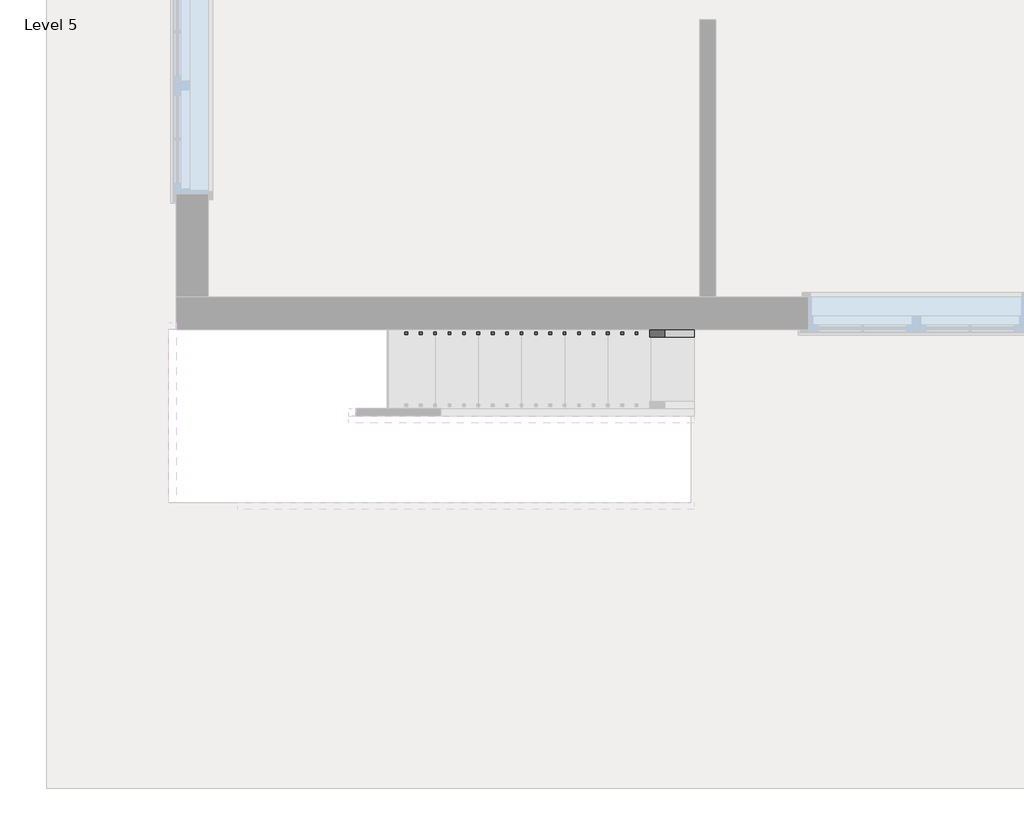
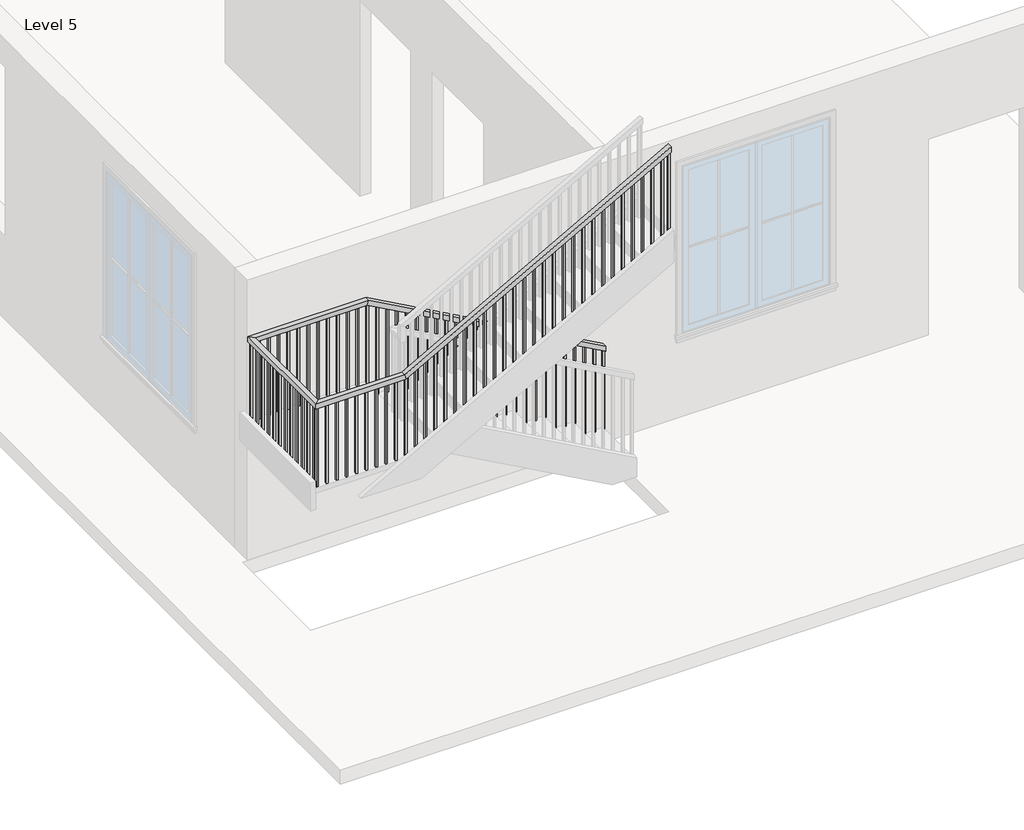
# One storey, part 2 of 3: 1 railing.
"""IFC4 building model written with IfcOpenShell, lengths in millimetres."""

from ifc_helpers import new_model, si_unit, frame, origin, place, context, project, spatial, polyline, outline, extrude, faceted_brep, element, save

model = new_model("IFC4")

# Units and contexts
model_context = context("Model", 3, world=origin())
ifc_project = project(units=[si_unit("LENGTHUNIT", "METRE", prefix="MILLI")], contexts=[model_context])

# Site, building, storey
site = spatial("IfcSite", under=ifc_project)
building = spatial("IfcBuilding", under=site)
storey = spatial("IfcBuildingStorey", under=building, Name="Level 5", Elevation=9601.2)

# Railing
placement = place(None, origin())
element("IfcRailing", 1, ObjectType="Handrail - Rectangular", at=placement, inside=storey, context=model_context, shape_type="SolidModel", body=[
    faceted_brep([(-1805.9198569, -5357.1933037, 10684.9333333), (-1805.9198569, -5357.1933037, 10626.820221), (-1805.9198569, -5306.3933037, 10626.820221), (-1805.9198569, -5306.3933037, 10684.9333333), (-4244.3198569, -5357.1933037, 12039.6), (-4257.4834592, -5357.1933037, 11988.8), (-4257.4834592, -5306.3933037, 11988.8), (-4244.3198569, -5306.3933037, 12039.6), (-5412.7198569, -5357.1933037, 12039.6), (-5412.7198569, -5357.1933037, 11988.8), (-5463.5198569, -5306.3933037, 11988.8), (-5463.5198569, -5306.3933037, 12039.6), (-5412.7198569, -6474.7933037, 12039.6), (-5412.7198569, -6474.7933037, 11988.8), (-5463.5198569, -6525.5933037, 11988.8), (-5463.5198569, -6525.5933037, 12039.6), (-4549.1198569, -6474.7933037, 12039.6), (-4535.9562547, -6474.7933037, 11988.8), (-4535.9562547, -6525.5933037, 11988.8), (-4549.1198569, -6525.5933037, 12039.6), (-1805.9198569, -6474.7933037, 13563.6), (-1805.9198569, -6525.5933037, 13563.6), (-1805.9198569, -6525.5933037, 13505.4868876), (-1805.9198569, -6474.7933037, 13505.4868876)], [[[0, 1, 2, 3]], [[1, 0, 4, 5]], [[2, 1, 5, 6]], [[3, 2, 6, 7]], [[0, 3, 7, 4]], [[5, 4, 8, 9]], [[6, 5, 9, 10]], [[7, 6, 10, 11]], [[4, 7, 11, 8]], [[9, 8, 12, 13]], [[10, 9, 13, 14]], [[11, 10, 14, 15]], [[8, 11, 15, 12]], [[13, 12, 16, 17]], [[14, 13, 17, 18]], [[15, 14, 18, 19]], [[12, 15, 19, 16]], [[20, 21, 22, 23]], [[17, 16, 20, 23]], [[18, 17, 23, 22]], [[19, 18, 22, 21]], [[16, 19, 21, 20]]]),
    extrude(outline(polyline([(13468.445221, -1872.5948569), (13457.8618876, -1891.6448569), (12479.8666667, -1891.6448569), (12479.8666667, -1872.5948569), (13468.445221, -1872.5948569)])), frame((0.0, -6509.7183037, 0.0), z_axis=(0.0, 1.0, 0.0), x_axis=(0.0, 0.0, 1.0)), (0.0, 0.0, 1.0), 19.05),
    extrude(outline(polyline([(13412.0007765, -1974.1948569), (13401.4174432, -1993.2448569), (12479.8666667, -1993.2448569), (12479.8666667, -1974.1948569), (13412.0007765, -1974.1948569)])), frame((0.0, -6509.7183037, 0.0), z_axis=(0.0, 1.0, 0.0), x_axis=(0.0, 0.0, 1.0)), (0.0, 0.0, 1.0), 19.05),
    extrude(outline(polyline([(13355.5563321, -2075.7948569), (13344.9729988, -2094.8448569), (12479.8666667, -2094.8448569), (12479.8666667, -2075.7948569), (13355.5563321, -2075.7948569)])), frame((0.0, -6509.7183037, 0.0), z_axis=(0.0, 1.0, 0.0), x_axis=(0.0, 0.0, 1.0)), (0.0, 0.0, 1.0), 19.05),
    extrude(outline(polyline([(13299.1118876, -2177.3948569), (13288.5285543, -2196.4448569), (12310.5333333, -2196.4448569), (12310.5333333, -2177.3948569), (13299.1118876, -2177.3948569)])), frame((0.0, -6509.7183037, 0.0), z_axis=(0.0, 1.0, 0.0), x_axis=(0.0, 0.0, 1.0)), (0.0, 0.0, 1.0), 19.05),
    extrude(outline(polyline([(13242.6674432, -2278.9948569), (13232.0841099, -2298.0448569), (12310.5333333, -2298.0448569), (12310.5333333, -2278.9948569), (13242.6674432, -2278.9948569)])), frame((0.0, -6509.7183037, 0.0), z_axis=(0.0, 1.0, 0.0), x_axis=(0.0, 0.0, 1.0)), (0.0, 0.0, 1.0), 19.05),
    extrude(outline(polyline([(13186.2229988, -2380.5948569), (13175.6396654, -2399.6448569), (12310.5333333, -2399.6448569), (12310.5333333, -2380.5948569), (13186.2229988, -2380.5948569)])), frame((0.0, -6509.7183037, 0.0), z_axis=(0.0, 1.0, 0.0), x_axis=(0.0, 0.0, 1.0)), (0.0, 0.0, 1.0), 19.05),
    extrude(outline(polyline([(13129.7785543, -2482.1948569), (13119.195221, -2501.2448569), (12141.2, -2501.2448569), (12141.2, -2482.1948569), (13129.7785543, -2482.1948569)])), frame((0.0, -6509.7183037, 0.0), z_axis=(0.0, 1.0, 0.0), x_axis=(0.0, 0.0, 1.0)), (0.0, 0.0, 1.0), 19.05),
    extrude(outline(polyline([(13073.3341099, -2583.7948569), (13062.7507765, -2602.8448569), (12141.2, -2602.8448569), (12141.2, -2583.7948569), (13073.3341099, -2583.7948569)])), frame((0.0, -6509.7183037, 0.0), z_axis=(0.0, 1.0, 0.0), x_axis=(0.0, 0.0, 1.0)), (0.0, 0.0, 1.0), 19.05),
    extrude(outline(polyline([(13016.8896654, -2685.3948569), (13006.3063321, -2704.4448569), (12141.2, -2704.4448569), (12141.2, -2685.3948569), (13016.8896654, -2685.3948569)])), frame((0.0, -6509.7183037, 0.0), z_axis=(0.0, 1.0, 0.0), x_axis=(0.0, 0.0, 1.0)), (0.0, 0.0, 1.0), 19.05),
    extrude(outline(polyline([(12960.445221, -2786.9948569), (12949.8618876, -2806.0448569), (11971.8666667, -2806.0448569), (11971.8666667, -2786.9948569), (12960.445221, -2786.9948569)])), frame((0.0, -6509.7183037, 0.0), z_axis=(0.0, 1.0, 0.0), x_axis=(0.0, 0.0, 1.0)), (0.0, 0.0, 1.0), 19.05),
    extrude(outline(polyline([(12904.0007765, -2888.5948569), (12893.4174432, -2907.6448569), (11971.8666667, -2907.6448569), (11971.8666667, -2888.5948569), (12904.0007765, -2888.5948569)])), frame((0.0, -6509.7183037, 0.0), z_axis=(0.0, 1.0, 0.0), x_axis=(0.0, 0.0, 1.0)), (0.0, 0.0, 1.0), 19.05),
    extrude(outline(polyline([(12847.5563321, -2990.1948569), (12836.9729988, -3009.2448569), (11971.8666667, -3009.2448569), (11971.8666667, -2990.1948569), (12847.5563321, -2990.1948569)])), frame((0.0, -6509.7183037, 0.0), z_axis=(0.0, 1.0, 0.0), x_axis=(0.0, 0.0, 1.0)), (0.0, 0.0, 1.0), 19.05),
    extrude(outline(polyline([(12791.1118876, -3091.7948569), (12780.5285543, -3110.8448569), (11802.5333333, -3110.8448569), (11802.5333333, -3091.7948569), (12791.1118876, -3091.7948569)])), frame((0.0, -6509.7183037, 0.0), z_axis=(0.0, 1.0, 0.0), x_axis=(0.0, 0.0, 1.0)), (0.0, 0.0, 1.0), 19.05),
    extrude(outline(polyline([(12734.6674432, -3193.3948569), (12724.0841099, -3212.4448569), (11802.5333333, -3212.4448569), (11802.5333333, -3193.3948569), (12734.6674432, -3193.3948569)])), frame((0.0, -6509.7183037, 0.0), z_axis=(0.0, 1.0, 0.0), x_axis=(0.0, 0.0, 1.0)), (0.0, 0.0, 1.0), 19.05),
    extrude(outline(polyline([(12678.2229988, -3294.9948569), (12667.6396654, -3314.0448569), (11802.5333333, -3314.0448569), (11802.5333333, -3294.9948569), (12678.2229988, -3294.9948569)])), frame((0.0, -6509.7183037, 0.0), z_axis=(0.0, 1.0, 0.0), x_axis=(0.0, 0.0, 1.0)), (0.0, 0.0, 1.0), 19.05),
    extrude(outline(polyline([(12621.7785543, -3396.5948569), (12611.195221, -3415.6448569), (11633.2, -3415.6448569), (11633.2, -3396.5948569), (12621.7785543, -3396.5948569)])), frame((0.0, -6509.7183037, 0.0), z_axis=(0.0, 1.0, 0.0), x_axis=(0.0, 0.0, 1.0)), (0.0, 0.0, 1.0), 19.05),
    extrude(outline(polyline([(12565.3341099, -3498.1948569), (12554.7507765, -3517.2448569), (11633.2, -3517.2448569), (11633.2, -3498.1948569), (12565.3341099, -3498.1948569)])), frame((0.0, -6509.7183037, 0.0), z_axis=(0.0, 1.0, 0.0), x_axis=(0.0, 0.0, 1.0)), (0.0, 0.0, 1.0), 19.05),
    extrude(outline(polyline([(12508.8896654, -3599.7948569), (12498.3063321, -3618.8448569), (11633.2, -3618.8448569), (11633.2, -3599.7948569), (12508.8896654, -3599.7948569)])), frame((0.0, -6509.7183037, 0.0), z_axis=(0.0, 1.0, 0.0), x_axis=(0.0, 0.0, 1.0)), (0.0, 0.0, 1.0), 19.05),
    extrude(outline(polyline([(12452.445221, -3701.3948569), (12441.8618876, -3720.4448569), (11463.8666667, -3720.4448569), (11463.8666667, -3701.3948569), (12452.445221, -3701.3948569)])), frame((0.0, -6509.7183037, 0.0), z_axis=(0.0, 1.0, 0.0), x_axis=(0.0, 0.0, 1.0)), (0.0, 0.0, 1.0), 19.05),
    extrude(outline(polyline([(12396.0007765, -3802.9948569), (12385.4174432, -3822.0448569), (11463.8666667, -3822.0448569), (11463.8666667, -3802.9948569), (12396.0007765, -3802.9948569)])), frame((0.0, -6509.7183037, 0.0), z_axis=(0.0, 1.0, 0.0), x_axis=(0.0, 0.0, 1.0)), (0.0, 0.0, 1.0), 19.05),
    extrude(outline(polyline([(12339.5563321, -3904.5948569), (12328.9729988, -3923.6448569), (11463.8666667, -3923.6448569), (11463.8666667, -3904.5948569), (12339.5563321, -3904.5948569)])), frame((0.0, -6509.7183037, 0.0), z_axis=(0.0, 1.0, 0.0), x_axis=(0.0, 0.0, 1.0)), (0.0, 0.0, 1.0), 19.05),
    extrude(outline(polyline([(12283.1118876, -4006.1948569), (12272.5285543, -4025.2448569), (11294.5333333, -4025.2448569), (11294.5333333, -4006.1948569), (12283.1118876, -4006.1948569)])), frame((0.0, -6509.7183037, 0.0), z_axis=(0.0, 1.0, 0.0), x_axis=(0.0, 0.0, 1.0)), (0.0, 0.0, 1.0), 19.05),
    extrude(outline(polyline([(12226.6674432, -4107.7948569), (12216.0841099, -4126.8448569), (11294.5333333, -4126.8448569), (11294.5333333, -4107.7948569), (12226.6674432, -4107.7948569)])), frame((0.0, -6509.7183037, 0.0), z_axis=(0.0, 1.0, 0.0), x_axis=(0.0, 0.0, 1.0)), (0.0, 0.0, 1.0), 19.05),
    extrude(outline(polyline([(12170.2229988, -4209.3948569), (12159.6396654, -4228.4448569), (11294.5333333, -4228.4448569), (11294.5333333, -4209.3948569), (12170.2229988, -4209.3948569)])), frame((0.0, -6509.7183037, 0.0), z_axis=(0.0, 1.0, 0.0), x_axis=(0.0, 0.0, 1.0)), (0.0, 0.0, 1.0), 19.05),
    extrude(outline(polyline([(12113.7785543, -4310.9948569), (12103.195221, -4330.0448569), (11125.2, -4330.0448569), (11125.2, -4310.9948569), (12113.7785543, -4310.9948569)])), frame((0.0, -6509.7183037, 0.0), z_axis=(0.0, 1.0, 0.0), x_axis=(0.0, 0.0, 1.0)), (0.0, 0.0, 1.0), 19.05),
    extrude(outline(polyline([(12057.3341099, -4412.5948569), (12046.7507765, -4431.6448569), (11125.2, -4431.6448569), (11125.2, -4412.5948569), (12057.3341099, -4412.5948569)])), frame((0.0, -6509.7183037, 0.0), z_axis=(0.0, 1.0, 0.0), x_axis=(0.0, 0.0, 1.0)), (0.0, 0.0, 1.0), 19.05),
    extrude(outline(polyline([(12000.8896654, -4514.1948569), (11990.3063321, -4533.2448569), (11125.2, -4533.2448569), (11125.2, -4514.1948569), (12000.8896654, -4514.1948569)])), frame((0.0, -6509.7183037, 0.0), z_axis=(0.0, 1.0, 0.0), x_axis=(0.0, 0.0, 1.0)), (0.0, 0.0, 1.0), 19.05),
    extrude(outline(polyline([(-4634.8448569, -6509.7183037), (-4634.8448569, -6490.6683037), (-4615.7948569, -6490.6683037), (-4615.7948569, -6509.7183037), (-4634.8448569, -6509.7183037)])), frame((0.0, 0.0, 11125.2), z_axis=(0.0, 0.0, 1.0), x_axis=(1.0, 0.0, 0.0)), (0.0, 0.0, 1.0), 863.6),
    extrude(outline(polyline([(-4736.4448569, -6509.7183037), (-4736.4448569, -6490.6683037), (-4717.3948569, -6490.6683037), (-4717.3948569, -6509.7183037), (-4736.4448569, -6509.7183037)])), frame((0.0, 0.0, 11125.2), z_axis=(0.0, 0.0, 1.0), x_axis=(1.0, 0.0, 0.0)), (0.0, 0.0, 1.0), 863.6),
    extrude(outline(polyline([(-4838.0448569, -6509.7183037), (-4838.0448569, -6490.6683037), (-4818.9948569, -6490.6683037), (-4818.9948569, -6509.7183037), (-4838.0448569, -6509.7183037)])), frame((0.0, 0.0, 11125.2), z_axis=(0.0, 0.0, 1.0), x_axis=(1.0, 0.0, 0.0)), (0.0, 0.0, 1.0), 863.6),
    extrude(outline(polyline([(-4939.6448569, -6509.7183037), (-4939.6448569, -6490.6683037), (-4920.5948569, -6490.6683037), (-4920.5948569, -6509.7183037), (-4939.6448569, -6509.7183037)])), frame((0.0, 0.0, 11125.2), z_axis=(0.0, 0.0, 1.0), x_axis=(1.0, 0.0, 0.0)), (0.0, 0.0, 1.0), 863.6),
    extrude(outline(polyline([(-5041.2448569, -6509.7183037), (-5041.2448569, -6490.6683037), (-5022.1948569, -6490.6683037), (-5022.1948569, -6509.7183037), (-5041.2448569, -6509.7183037)])), frame((0.0, 0.0, 11125.2), z_axis=(0.0, 0.0, 1.0), x_axis=(1.0, 0.0, 0.0)), (0.0, 0.0, 1.0), 863.6),
    extrude(outline(polyline([(-5142.8448569, -6509.7183037), (-5142.8448569, -6490.6683037), (-5123.7948569, -6490.6683037), (-5123.7948569, -6509.7183037), (-5142.8448569, -6509.7183037)])), frame((0.0, 0.0, 11125.2), z_axis=(0.0, 0.0, 1.0), x_axis=(1.0, 0.0, 0.0)), (0.0, 0.0, 1.0), 863.6),
    extrude(outline(polyline([(-5244.4448569, -6509.7183037), (-5244.4448569, -6490.6683037), (-5225.3948569, -6490.6683037), (-5225.3948569, -6509.7183037), (-5244.4448569, -6509.7183037)])), frame((0.0, 0.0, 11125.2), z_axis=(0.0, 0.0, 1.0), x_axis=(1.0, 0.0, 0.0)), (0.0, 0.0, 1.0), 863.6),
    extrude(outline(polyline([(-5346.0448569, -6509.7183037), (-5346.0448569, -6490.6683037), (-5326.9948569, -6490.6683037), (-5326.9948569, -6509.7183037), (-5346.0448569, -6509.7183037)])), frame((0.0, 0.0, 11125.2), z_axis=(0.0, 0.0, 1.0), x_axis=(1.0, 0.0, 0.0)), (0.0, 0.0, 1.0), 863.6),
    extrude(outline(polyline([(-5447.6448569, -6439.8683037), (-5428.5948569, -6439.8683037), (-5428.5948569, -6458.9183037), (-5447.6448569, -6458.9183037), (-5447.6448569, -6439.8683037)])), frame((0.0, 0.0, 11125.2), z_axis=(0.0, 0.0, 1.0), x_axis=(1.0, 0.0, 0.0)), (0.0, 0.0, 1.0), 863.6),
    extrude(outline(polyline([(-5447.6448569, -6338.2683037), (-5428.5948569, -6338.2683037), (-5428.5948569, -6357.3183037), (-5447.6448569, -6357.3183037), (-5447.6448569, -6338.2683037)])), frame((0.0, 0.0, 11125.2), z_axis=(0.0, 0.0, 1.0), x_axis=(1.0, 0.0, 0.0)), (0.0, 0.0, 1.0), 863.6),
    extrude(outline(polyline([(-5447.6448569, -6236.6683037), (-5428.5948569, -6236.6683037), (-5428.5948569, -6255.7183037), (-5447.6448569, -6255.7183037), (-5447.6448569, -6236.6683037)])), frame((0.0, 0.0, 11125.2), z_axis=(0.0, 0.0, 1.0), x_axis=(1.0, 0.0, 0.0)), (0.0, 0.0, 1.0), 863.6),
    extrude(outline(polyline([(-5447.6448569, -6135.0683037), (-5428.5948569, -6135.0683037), (-5428.5948569, -6154.1183037), (-5447.6448569, -6154.1183037), (-5447.6448569, -6135.0683037)])), frame((0.0, 0.0, 11125.2), z_axis=(0.0, 0.0, 1.0), x_axis=(1.0, 0.0, 0.0)), (0.0, 0.0, 1.0), 863.6),
    extrude(outline(polyline([(-5447.6448569, -6033.4683037), (-5428.5948569, -6033.4683037), (-5428.5948569, -6052.5183037), (-5447.6448569, -6052.5183037), (-5447.6448569, -6033.4683037)])), frame((0.0, 0.0, 11125.2), z_axis=(0.0, 0.0, 1.0), x_axis=(1.0, 0.0, 0.0)), (0.0, 0.0, 1.0), 863.6),
    extrude(outline(polyline([(-5447.6448569, -5931.8683037), (-5428.5948569, -5931.8683037), (-5428.5948569, -5950.9183037), (-5447.6448569, -5950.9183037), (-5447.6448569, -5931.8683037)])), frame((0.0, 0.0, 11125.2), z_axis=(0.0, 0.0, 1.0), x_axis=(1.0, 0.0, 0.0)), (0.0, 0.0, 1.0), 863.6),
    extrude(outline(polyline([(-5447.6448569, -5830.2683037), (-5428.5948569, -5830.2683037), (-5428.5948569, -5849.3183037), (-5447.6448569, -5849.3183037), (-5447.6448569, -5830.2683037)])), frame((0.0, 0.0, 11125.2), z_axis=(0.0, 0.0, 1.0), x_axis=(1.0, 0.0, 0.0)), (0.0, 0.0, 1.0), 863.6),
    extrude(outline(polyline([(-5447.6448569, -5728.6683037), (-5428.5948569, -5728.6683037), (-5428.5948569, -5747.7183037), (-5447.6448569, -5747.7183037), (-5447.6448569, -5728.6683037)])), frame((0.0, 0.0, 11125.2), z_axis=(0.0, 0.0, 1.0), x_axis=(1.0, 0.0, 0.0)), (0.0, 0.0, 1.0), 863.6),
    extrude(outline(polyline([(-5447.6448569, -5627.0683037), (-5428.5948569, -5627.0683037), (-5428.5948569, -5646.1183037), (-5447.6448569, -5646.1183037), (-5447.6448569, -5627.0683037)])), frame((0.0, 0.0, 11125.2), z_axis=(0.0, 0.0, 1.0), x_axis=(1.0, 0.0, 0.0)), (0.0, 0.0, 1.0), 863.6),
    extrude(outline(polyline([(-5447.6448569, -5525.4683037), (-5428.5948569, -5525.4683037), (-5428.5948569, -5544.5183037), (-5447.6448569, -5544.5183037), (-5447.6448569, -5525.4683037)])), frame((0.0, 0.0, 11125.2), z_axis=(0.0, 0.0, 1.0), x_axis=(1.0, 0.0, 0.0)), (0.0, 0.0, 1.0), 863.6),
    extrude(outline(polyline([(-5447.6448569, -5423.8683037), (-5428.5948569, -5423.8683037), (-5428.5948569, -5442.9183037), (-5447.6448569, -5442.9183037), (-5447.6448569, -5423.8683037)])), frame((0.0, 0.0, 11125.2), z_axis=(0.0, 0.0, 1.0), x_axis=(1.0, 0.0, 0.0)), (0.0, 0.0, 1.0), 863.6),
    extrude(outline(polyline([(-5352.3948569, -5322.2683037), (-5352.3948569, -5341.3183037), (-5371.4448569, -5341.3183037), (-5371.4448569, -5322.2683037), (-5352.3948569, -5322.2683037)])), frame((0.0, 0.0, 11125.2), z_axis=(0.0, 0.0, 1.0), x_axis=(1.0, 0.0, 0.0)), (0.0, 0.0, 1.0), 863.6),
    extrude(outline(polyline([(-5250.7948569, -5322.2683037), (-5250.7948569, -5341.3183037), (-5269.8448569, -5341.3183037), (-5269.8448569, -5322.2683037), (-5250.7948569, -5322.2683037)])), frame((0.0, 0.0, 11125.2), z_axis=(0.0, 0.0, 1.0), x_axis=(1.0, 0.0, 0.0)), (0.0, 0.0, 1.0), 863.6),
    extrude(outline(polyline([(-5149.1948569, -5322.2683037), (-5149.1948569, -5341.3183037), (-5168.2448569, -5341.3183037), (-5168.2448569, -5322.2683037), (-5149.1948569, -5322.2683037)])), frame((0.0, 0.0, 11125.2), z_axis=(0.0, 0.0, 1.0), x_axis=(1.0, 0.0, 0.0)), (0.0, 0.0, 1.0), 863.6),
    extrude(outline(polyline([(-5047.5948569, -5322.2683037), (-5047.5948569, -5341.3183037), (-5066.6448569, -5341.3183037), (-5066.6448569, -5322.2683037), (-5047.5948569, -5322.2683037)])), frame((0.0, 0.0, 11125.2), z_axis=(0.0, 0.0, 1.0), x_axis=(1.0, 0.0, 0.0)), (0.0, 0.0, 1.0), 863.6),
    extrude(outline(polyline([(-4945.9948569, -5322.2683037), (-4945.9948569, -5341.3183037), (-4965.0448569, -5341.3183037), (-4965.0448569, -5322.2683037), (-4945.9948569, -5322.2683037)])), frame((0.0, 0.0, 11125.2), z_axis=(0.0, 0.0, 1.0), x_axis=(1.0, 0.0, 0.0)), (0.0, 0.0, 1.0), 863.6),
    extrude(outline(polyline([(-4844.3948569, -5322.2683037), (-4844.3948569, -5341.3183037), (-4863.4448569, -5341.3183037), (-4863.4448569, -5322.2683037), (-4844.3948569, -5322.2683037)])), frame((0.0, 0.0, 11125.2), z_axis=(0.0, 0.0, 1.0), x_axis=(1.0, 0.0, 0.0)), (0.0, 0.0, 1.0), 863.6),
    extrude(outline(polyline([(-4742.7948569, -5322.2683037), (-4742.7948569, -5341.3183037), (-4761.8448569, -5341.3183037), (-4761.8448569, -5322.2683037), (-4742.7948569, -5322.2683037)])), frame((0.0, 0.0, 11125.2), z_axis=(0.0, 0.0, 1.0), x_axis=(1.0, 0.0, 0.0)), (0.0, 0.0, 1.0), 863.6),
    extrude(outline(polyline([(-4641.1948569, -5322.2683037), (-4641.1948569, -5341.3183037), (-4660.2448569, -5341.3183037), (-4660.2448569, -5322.2683037), (-4641.1948569, -5322.2683037)])), frame((0.0, 0.0, 11125.2), z_axis=(0.0, 0.0, 1.0), x_axis=(1.0, 0.0, 0.0)), (0.0, 0.0, 1.0), 863.6),
    extrude(outline(polyline([(-4539.5948569, -5322.2683037), (-4539.5948569, -5341.3183037), (-4558.6448569, -5341.3183037), (-4558.6448569, -5322.2683037), (-4539.5948569, -5322.2683037)])), frame((0.0, 0.0, 11125.2), z_axis=(0.0, 0.0, 1.0), x_axis=(1.0, 0.0, 0.0)), (0.0, 0.0, 1.0), 863.6),
    extrude(outline(polyline([(-4437.9948569, -5322.2683037), (-4437.9948569, -5341.3183037), (-4457.0448569, -5341.3183037), (-4457.0448569, -5322.2683037), (-4437.9948569, -5322.2683037)])), frame((0.0, 0.0, 11125.2), z_axis=(0.0, 0.0, 1.0), x_axis=(1.0, 0.0, 0.0)), (0.0, 0.0, 1.0), 863.6),
    extrude(outline(polyline([(-4336.3948569, -5322.2683037), (-4336.3948569, -5341.3183037), (-4355.4448569, -5341.3183037), (-4355.4448569, -5322.2683037), (-4336.3948569, -5322.2683037)])), frame((0.0, 0.0, 11125.2), z_axis=(0.0, 0.0, 1.0), x_axis=(1.0, 0.0, 0.0)), (0.0, 0.0, 1.0), 863.6),
    extrude(outline(polyline([(11976.195221, -4234.7948569), (11986.7785543, -4253.8448569), (11125.2, -4253.8448569), (11125.2, -4234.7948569), (11976.195221, -4234.7948569)])), frame((0.0, -5341.3183037, 0.0), z_axis=(0.0, 1.0, 0.0), x_axis=(0.0, 0.0, 1.0)), (0.0, 0.0, 1.0), 19.05),
    extrude(outline(polyline([(11919.7507765, -4133.1948569), (11930.3341099, -4152.2448569), (10955.8666667, -4152.2448569), (10955.8666667, -4133.1948569), (11919.7507765, -4133.1948569)])), frame((0.0, -5341.3183037, 0.0), z_axis=(0.0, 1.0, 0.0), x_axis=(0.0, 0.0, 1.0)), (0.0, 0.0, 1.0), 19.05),
    extrude(outline(polyline([(11863.3063321, -4031.5948569), (11873.8896654, -4050.6448569), (10955.8666667, -4050.6448569), (10955.8666667, -4031.5948569), (11863.3063321, -4031.5948569)])), frame((0.0, -5341.3183037, 0.0), z_axis=(0.0, 1.0, 0.0), x_axis=(0.0, 0.0, 1.0)), (0.0, 0.0, 1.0), 19.05),
    extrude(outline(polyline([(11806.8618876, -3929.9948569), (11817.445221, -3949.0448569), (10955.8666667, -3949.0448569), (10955.8666667, -3929.9948569), (11806.8618876, -3929.9948569)])), frame((0.0, -5341.3183037, 0.0), z_axis=(0.0, 1.0, 0.0), x_axis=(0.0, 0.0, 1.0)), (0.0, 0.0, 1.0), 19.05),
    extrude(outline(polyline([(11750.4174432, -3828.3948569), (11761.0007765, -3847.4448569), (10786.5333333, -3847.4448569), (10786.5333333, -3828.3948569), (11750.4174432, -3828.3948569)])), frame((0.0, -5341.3183037, 0.0), z_axis=(0.0, 1.0, 0.0), x_axis=(0.0, 0.0, 1.0)), (0.0, 0.0, 1.0), 19.05),
    extrude(outline(polyline([(11693.9729988, -3726.7948569), (11704.5563321, -3745.8448569), (10786.5333333, -3745.8448569), (10786.5333333, -3726.7948569), (11693.9729988, -3726.7948569)])), frame((0.0, -5341.3183037, 0.0), z_axis=(0.0, 1.0, 0.0), x_axis=(0.0, 0.0, 1.0)), (0.0, 0.0, 1.0), 19.05),
    extrude(outline(polyline([(11637.5285543, -3625.1948569), (11648.1118876, -3644.2448569), (10786.5333333, -3644.2448569), (10786.5333333, -3625.1948569), (11637.5285543, -3625.1948569)])), frame((0.0, -5341.3183037, 0.0), z_axis=(0.0, 1.0, 0.0), x_axis=(0.0, 0.0, 1.0)), (0.0, 0.0, 1.0), 19.05),
    extrude(outline(polyline([(11581.0841099, -3523.5948569), (11591.6674432, -3542.6448569), (10617.2, -3542.6448569), (10617.2, -3523.5948569), (11581.0841099, -3523.5948569)])), frame((0.0, -5341.3183037, 0.0), z_axis=(0.0, 1.0, 0.0), x_axis=(0.0, 0.0, 1.0)), (0.0, 0.0, 1.0), 19.05),
    extrude(outline(polyline([(11524.6396654, -3421.9948569), (11535.2229988, -3441.0448569), (10617.2, -3441.0448569), (10617.2, -3421.9948569), (11524.6396654, -3421.9948569)])), frame((0.0, -5341.3183037, 0.0), z_axis=(0.0, 1.0, 0.0), x_axis=(0.0, 0.0, 1.0)), (0.0, 0.0, 1.0), 19.05),
    extrude(outline(polyline([(11468.195221, -3320.3948569), (11478.7785543, -3339.4448569), (10617.2, -3339.4448569), (10617.2, -3320.3948569), (11468.195221, -3320.3948569)])), frame((0.0, -5341.3183037, 0.0), z_axis=(0.0, 1.0, 0.0), x_axis=(0.0, 0.0, 1.0)), (0.0, 0.0, 1.0), 19.05),
    extrude(outline(polyline([(11411.7507765, -3218.7948569), (11422.3341099, -3237.8448569), (10447.8666667, -3237.8448569), (10447.8666667, -3218.7948569), (11411.7507765, -3218.7948569)])), frame((0.0, -5341.3183037, 0.0), z_axis=(0.0, 1.0, 0.0), x_axis=(0.0, 0.0, 1.0)), (0.0, 0.0, 1.0), 19.05),
    extrude(outline(polyline([(11355.3063321, -3117.1948569), (11365.8896654, -3136.2448569), (10447.8666667, -3136.2448569), (10447.8666667, -3117.1948569), (11355.3063321, -3117.1948569)])), frame((0.0, -5341.3183037, 0.0), z_axis=(0.0, 1.0, 0.0), x_axis=(0.0, 0.0, 1.0)), (0.0, 0.0, 1.0), 19.05),
    extrude(outline(polyline([(11298.8618876, -3015.5948569), (11309.445221, -3034.6448569), (10447.8666667, -3034.6448569), (10447.8666667, -3015.5948569), (11298.8618876, -3015.5948569)])), frame((0.0, -5341.3183037, 0.0), z_axis=(0.0, 1.0, 0.0), x_axis=(0.0, 0.0, 1.0)), (0.0, 0.0, 1.0), 19.05),
    extrude(outline(polyline([(11242.4174432, -2913.9948569), (11253.0007765, -2933.0448569), (10278.5333333, -2933.0448569), (10278.5333333, -2913.9948569), (11242.4174432, -2913.9948569)])), frame((0.0, -5341.3183037, 0.0), z_axis=(0.0, 1.0, 0.0), x_axis=(0.0, 0.0, 1.0)), (0.0, 0.0, 1.0), 19.05),
    extrude(outline(polyline([(11185.9729988, -2812.3948569), (11196.5563321, -2831.4448569), (10278.5333333, -2831.4448569), (10278.5333333, -2812.3948569), (11185.9729988, -2812.3948569)])), frame((0.0, -5341.3183037, 0.0), z_axis=(0.0, 1.0, 0.0), x_axis=(0.0, 0.0, 1.0)), (0.0, 0.0, 1.0), 19.05),
    extrude(outline(polyline([(11129.5285543, -2710.7948569), (11140.1118876, -2729.8448569), (10278.5333333, -2729.8448569), (10278.5333333, -2710.7948569), (11129.5285543, -2710.7948569)])), frame((0.0, -5341.3183037, 0.0), z_axis=(0.0, 1.0, 0.0), x_axis=(0.0, 0.0, 1.0)), (0.0, 0.0, 1.0), 19.05),
    extrude(outline(polyline([(11073.0841099, -2609.1948569), (11083.6674432, -2628.2448569), (10109.2, -2628.2448569), (10109.2, -2609.1948569), (11073.0841099, -2609.1948569)])), frame((0.0, -5341.3183037, 0.0), z_axis=(0.0, 1.0, 0.0), x_axis=(0.0, 0.0, 1.0)), (0.0, 0.0, 1.0), 19.05),
    extrude(outline(polyline([(11016.6396654, -2507.5948569), (11027.2229988, -2526.6448569), (10109.2, -2526.6448569), (10109.2, -2507.5948569), (11016.6396654, -2507.5948569)])), frame((0.0, -5341.3183037, 0.0), z_axis=(0.0, 1.0, 0.0), x_axis=(0.0, 0.0, 1.0)), (0.0, 0.0, 1.0), 19.05),
    extrude(outline(polyline([(10960.195221, -2405.9948569), (10970.7785543, -2425.0448569), (10109.2, -2425.0448569), (10109.2, -2405.9948569), (10960.195221, -2405.9948569)])), frame((0.0, -5341.3183037, 0.0), z_axis=(0.0, 1.0, 0.0), x_axis=(0.0, 0.0, 1.0)), (0.0, 0.0, 1.0), 19.05),
    extrude(outline(polyline([(10903.7507765, -2304.3948569), (10914.3341099, -2323.4448569), (9939.8666667, -2323.4448569), (9939.8666667, -2304.3948569), (10903.7507765, -2304.3948569)])), frame((0.0, -5341.3183037, 0.0), z_axis=(0.0, 1.0, 0.0), x_axis=(0.0, 0.0, 1.0)), (0.0, 0.0, 1.0), 19.05),
    extrude(outline(polyline([(10847.3063321, -2202.7948569), (10857.8896654, -2221.8448569), (9939.8666667, -2221.8448569), (9939.8666667, -2202.7948569), (10847.3063321, -2202.7948569)])), frame((0.0, -5341.3183037, 0.0), z_axis=(0.0, 1.0, 0.0), x_axis=(0.0, 0.0, 1.0)), (0.0, 0.0, 1.0), 19.05),
    extrude(outline(polyline([(10790.8618876, -2101.1948569), (10801.445221, -2120.2448569), (9939.8666667, -2120.2448569), (9939.8666667, -2101.1948569), (10790.8618876, -2101.1948569)])), frame((0.0, -5341.3183037, 0.0), z_axis=(0.0, 1.0, 0.0), x_axis=(0.0, 0.0, 1.0)), (0.0, 0.0, 1.0), 19.05),
    extrude(outline(polyline([(10734.4174432, -1999.5948569), (10745.0007765, -2018.6448569), (9770.5333333, -2018.6448569), (9770.5333333, -1999.5948569), (10734.4174432, -1999.5948569)])), frame((0.0, -5341.3183037, 0.0), z_axis=(0.0, 1.0, 0.0), x_axis=(0.0, 0.0, 1.0)), (0.0, 0.0, 1.0), 19.05),
    extrude(outline(polyline([(10677.9729988, -1897.9948569), (10688.5563321, -1917.0448569), (9770.5333333, -1917.0448569), (9770.5333333, -1897.9948569), (10677.9729988, -1897.9948569)])), frame((0.0, -5341.3183037, 0.0), z_axis=(0.0, 1.0, 0.0), x_axis=(0.0, 0.0, 1.0)), (0.0, 0.0, 1.0), 19.05),
    extrude(outline(polyline([(-5447.6448569, -6490.6683037), (-5428.5948569, -6490.6683037), (-5428.5948569, -6509.7183037), (-5447.6448569, -6509.7183037), (-5447.6448569, -6490.6683037)])), frame((0.0, 0.0, 11125.2), z_axis=(0.0, 0.0, 1.0), x_axis=(1.0, 0.0, 0.0)), (0.0, 0.0, 1.0), 863.6),
    extrude(outline(polyline([(-5428.5948569, -5322.2683037), (-5428.5948569, -5341.3183037), (-5447.6448569, -5341.3183037), (-5447.6448569, -5322.2683037), (-5428.5948569, -5322.2683037)])), frame((0.0, 0.0, 11125.2), z_axis=(0.0, 0.0, 1.0), x_axis=(1.0, 0.0, 0.0)), (0.0, 0.0, 1.0), 863.6),
    extrude(outline(polyline([(13505.4868876, -1805.9198569), (13494.9035543, -1824.9698569), (12479.8666667, -1824.9698569), (12479.8666667, -1805.9198569), (13505.4868876, -1805.9198569)])), frame((0.0, -6509.7183037, 0.0), z_axis=(0.0, 1.0, 0.0), x_axis=(0.0, 0.0, 1.0)), (0.0, 0.0, 1.0), 19.05),
    extrude(outline(polyline([(10626.820221, -1805.9198569), (10637.4035543, -1824.9698569), (9770.5333333, -1824.9698569), (9770.5333333, -1805.9198569), (10626.820221, -1805.9198569)])), frame((0.0, -5341.3183037, 0.0), z_axis=(0.0, 1.0, 0.0), x_axis=(0.0, 0.0, 1.0)), (0.0, 0.0, 1.0), 19.05),
])

save(model, "model.ifc")

# Revit data of these elements
# Type "Handrail - Rectangular"
#   Assembly Code = "C2010400"
#   built-in parameter 1008612 = 0.0416667 (stored number, unit not read)
#   built-in parameter 1008611 = 0.0416667 (stored number, unit not read)
#   built-in parameter 1008609 = 0.333333 (stored number, unit not read)
#   built-in parameter 1008604 = 0.166667 (stored number, unit not read)
#   built-in parameter 1008603 = 0.166667 (stored number, unit not read)
#   Railing Height = 3' - 0"
#   built-in parameter 1008630 = 2
#   built-in parameter 1008610 = 2
#   built-in parameter 1008618 = Baluster - Square : 3/4"
# Element 1 (IfcRailing, "Handrail - Rectangular")
#   Phase Created = New Construction
